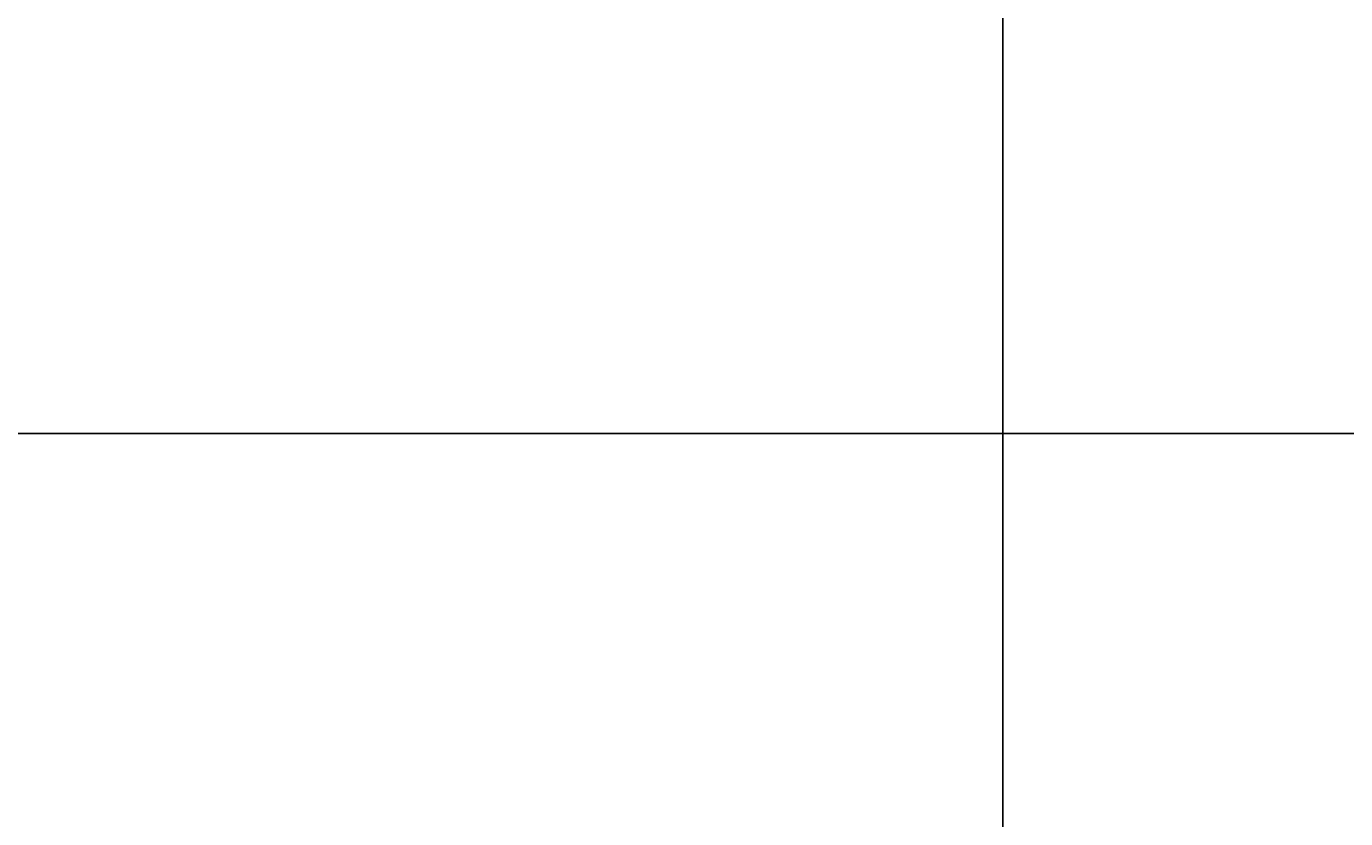
# Model space of a CAD drawing. Units: inches. Extents: x -301 to 715, y -607 to 364.
# Tile 14 of 141: x 18 to 59, y -524 to -499. Entities that reach past the tile are written whole.
import ezdxf

# ---------------------------------------------------------------- set-up
doc = ezdxf.new("R2010")
doc.units = ezdxf.units.IN
doc.header["$MEASUREMENT"] = 0
doc.layers.add('A-ANNO-DIMS', color=2, linetype='Continuous', lineweight=18)
doc.styles.get("Standard").update_dxf_attribs({"font": 'arial.ttf'})
doc.dimstyles.get("Standard").update_dxf_attribs({"dimtxt": 0.18, "dimasz": 0.18, "dimexe": 0.18, "dimexo": 0.0625, "dimgap": 0.09, "dimtad": 0, "dimtih": 1, "dimtoh": 1, "dimdec": 1, "dimzin": 0, "dimdsep": 46, "dimlunit": 4, "dimtxsty": 'Standard', "dimcen": 0.09, "dimclrd": 3, "dimclre": 4, "dimclrt": 6, "dimadec": 0, "dimazin": 0, "dimtfac": 1, "dimtdec": 1, "dimtofl": 0, "dimtmove": 0, "dimatfit": 3, "dimfxl": 1, "dimtfill": 2, "dimtfillclr": 51, "dimtolj": 1, "dimtzin": 0, "dimarcsym": 0})

# ---------------------------------------------------------------- blocks, each defined once
blk = doc.blocks.new('*D176')
at = {"layer": 'A-ANNO-DIMS', "color": 4, "lineweight": -2, "transparency": 16777216}
for p, q in [((148.28, -324.477), (215.605, -324.477)), ((-15.22, -540.477), (215.605, -540.477))]:
    blk.add_line(p, q, dxfattribs=at)
at = {"layer": 'A-ANNO-DIMS', "color": 3, "lineweight": -2, "transparency": 16777216}
for p, q in [((215.425, -324.657), (215.425, -432.296)), ((215.425, -540.297), (215.425, -432.659))]:
    blk.add_line(p, q, dxfattribs=at)
at = {"layer": 'A-ANNO-DIMS', "color": 3, "transparency": 16777216}
for points in [[(215.395, -324.657), (215.455, -324.657), (215.425, -324.477)], [(215.395, -540.297), (215.455, -540.297), (215.425, -540.477)]]:
    blk.add_solid(points, dxfattribs=at)
at = {"layer": 'Defpoints', "color": 0, "transparency": 16777216}
for p in [(148.218, -324.477), (-15.282, -540.477), (215.425, -540.477)]:
    blk.add_point(p, dxfattribs=at)
at = {"layer": 'A-ANNO-DIMS', "color": 6, "transparency": 16777216, "insert": (215.425, -432.477), "char_height": 0.18, "attachment_point": 5, "bg_fill": 1, "box_fill_scale": 1.25, "bg_fill_color": 51, "bg_fill_transparency": 0}
blk.add_mtext('\\A1;18\'-0"', dxfattribs=at)
blk = doc.blocks.new('*D181')
at = {"layer": 'A-ANNO-DIMS', "color": 4, "lineweight": -2, "transparency": 16777216}
for p, q in [((48.468, -433.54), (48.468, -573.809)), ((12.718, -463.54), (12.718, -573.809))]:
    blk.add_line(p, q, dxfattribs=at)
at = {"layer": 'A-ANNO-DIMS', "color": 3, "lineweight": -2, "transparency": 16777216}
for p, q in [((12.898, -573.629), (30.264, -573.629)), ((48.288, -573.629), (30.922, -573.629))]:
    blk.add_line(p, q, dxfattribs=at)
at = {"layer": 'A-ANNO-DIMS', "color": 3, "transparency": 16777216}
for points in [[(12.898, -573.599), (12.898, -573.659), (12.718, -573.629)], [(48.288, -573.599), (48.288, -573.659), (48.468, -573.629)]]:
    blk.add_solid(points, dxfattribs=at)
at = {"layer": 'Defpoints', "color": 0, "transparency": 16777216}
for p in [(48.468, -433.477), (12.718, -463.477), (48.468, -573.629)]:
    blk.add_point(p, dxfattribs=at)
at = {"layer": 'A-ANNO-DIMS', "color": 6, "transparency": 16777216, "insert": (30.593, -573.629), "char_height": 0.18, "attachment_point": 5, "bg_fill": 1, "box_fill_scale": 1.25, "bg_fill_color": 51, "bg_fill_transparency": 0}
blk.add_mtext('\\A1;3\'-0"', dxfattribs=at)
blk = doc.blocks.new('*D190')
at = {"layer": 'A-ANNO-DIMS', "color": 4, "lineweight": -2, "transparency": 16777216}
for p, q in [((129.193, -481.477), (-266.112, -481.477)), ((124.193, -511.477), (-266.112, -511.477))]:
    blk.add_line(p, q, dxfattribs=at)
at = {"layer": 'A-ANNO-DIMS', "color": 3, "lineweight": -2, "transparency": 16777216}
for p, q in [((-265.932, -481.657), (-265.932, -496.296)), ((-265.932, -511.297), (-265.932, -496.659))]:
    blk.add_line(p, q, dxfattribs=at)
at = {"layer": 'A-ANNO-DIMS', "color": 3, "transparency": 16777216}
for points in [[(-265.962, -481.657), (-265.902, -481.657), (-265.932, -481.477)], [(-265.962, -511.297), (-265.902, -511.297), (-265.932, -511.477)]]:
    blk.add_solid(points, dxfattribs=at)
at = {"layer": 'Defpoints', "color": 0, "transparency": 16777216}
for p in [(129.255, -481.477), (-265.932, -511.477), (124.255, -511.477)]:
    blk.add_point(p, dxfattribs=at)
at = {"layer": 'A-ANNO-DIMS', "color": 6, "transparency": 16777216, "insert": (-265.932, -496.477), "char_height": 0.18, "attachment_point": 5, "bg_fill": 1, "box_fill_scale": 1.25, "bg_fill_color": 51, "bg_fill_transparency": 0}
blk.add_mtext('\\A1;2\'-6"', dxfattribs=at)
blk = doc.blocks.new('*D191')
at = {"layer": 'A-ANNO-DIMS', "color": 4, "lineweight": -2, "transparency": 16777216}
for p, q in [((129.193, -481.477), (-266.112, -481.477)), ((114.193, -540.477), (-266.112, -540.477))]:
    blk.add_line(p, q, dxfattribs=at)
at = {"layer": 'A-ANNO-DIMS', "color": 3, "lineweight": -2, "transparency": 16777216}
for p, q in [((-265.932, -481.657), (-265.932, -510.797)), ((-265.932, -540.297), (-265.932, -511.158))]:
    blk.add_line(p, q, dxfattribs=at)
at = {"layer": 'A-ANNO-DIMS', "color": 3, "transparency": 16777216}
for points in [[(-265.962, -481.657), (-265.902, -481.657), (-265.932, -481.477)], [(-265.962, -540.297), (-265.902, -540.297), (-265.932, -540.477)]]:
    blk.add_solid(points, dxfattribs=at)
at = {"layer": 'Defpoints', "color": 0, "transparency": 16777216}
for p in [(129.255, -481.477), (-265.932, -540.477), (114.255, -540.477)]:
    blk.add_point(p, dxfattribs=at)
at = {"layer": 'A-ANNO-DIMS', "color": 6, "transparency": 16777216, "insert": (-265.932, -510.977), "char_height": 0.18, "attachment_point": 5, "bg_fill": 1, "box_fill_scale": 1.25, "bg_fill_color": 51, "bg_fill_transparency": 0}
blk.add_mtext('\\A1;4\'-11"', dxfattribs=at)

msp = doc.modelspace()

# ---------------------------------------------------------------- dimensions: what is measured, and where the dimension line sits
at = {"layer": 'A-ANNO-DIMS'}
for base, p1, p2, picture, middle in [((215.425, -540.477), (148.218, -324.477), (-15.282, -540.477), '*D176', (215.425, -432.477)), ((-265.932, -540.477), (129.255, -481.477), (114.255, -540.477), '*D191', (-265.932, -510.977)), ((-265.932, -511.477), (129.255, -481.477), (124.255, -511.477), '*D190', (-265.932, -496.477))]:
    dim = msp.add_linear_dim(base=base, p1=p1, p2=p2, angle=90, dimstyle='Standard', override={"dimdec": 1, "dimlfac": 1, "dimrnd": 0, "dimzin": 1, "dimdsep": 46, "dimlunit": 4, "dimfrac": 2}, dxfattribs=at)
    dim.commit()
    dim.dimension.update_dxf_attribs({"geometry": picture, "text_midpoint": middle})
dim = msp.add_linear_dim(base=(48.467984, -573.628877), p1=(12.717984, -463.47741), p2=(48.467984, -433.47741), dimstyle='Standard', override={"dimdec": 1, "dimlfac": 1, "dimrnd": 0, "dimzin": 1, "dimdsep": 46, "dimlunit": 4, "dimfrac": 2}, dxfattribs=at)
dim.commit()
dim.dimension.update_dxf_attribs({"geometry": '*D181', "text_midpoint": (30.592984, -573.628877)})

doc.saveas('drawing.dxf')
